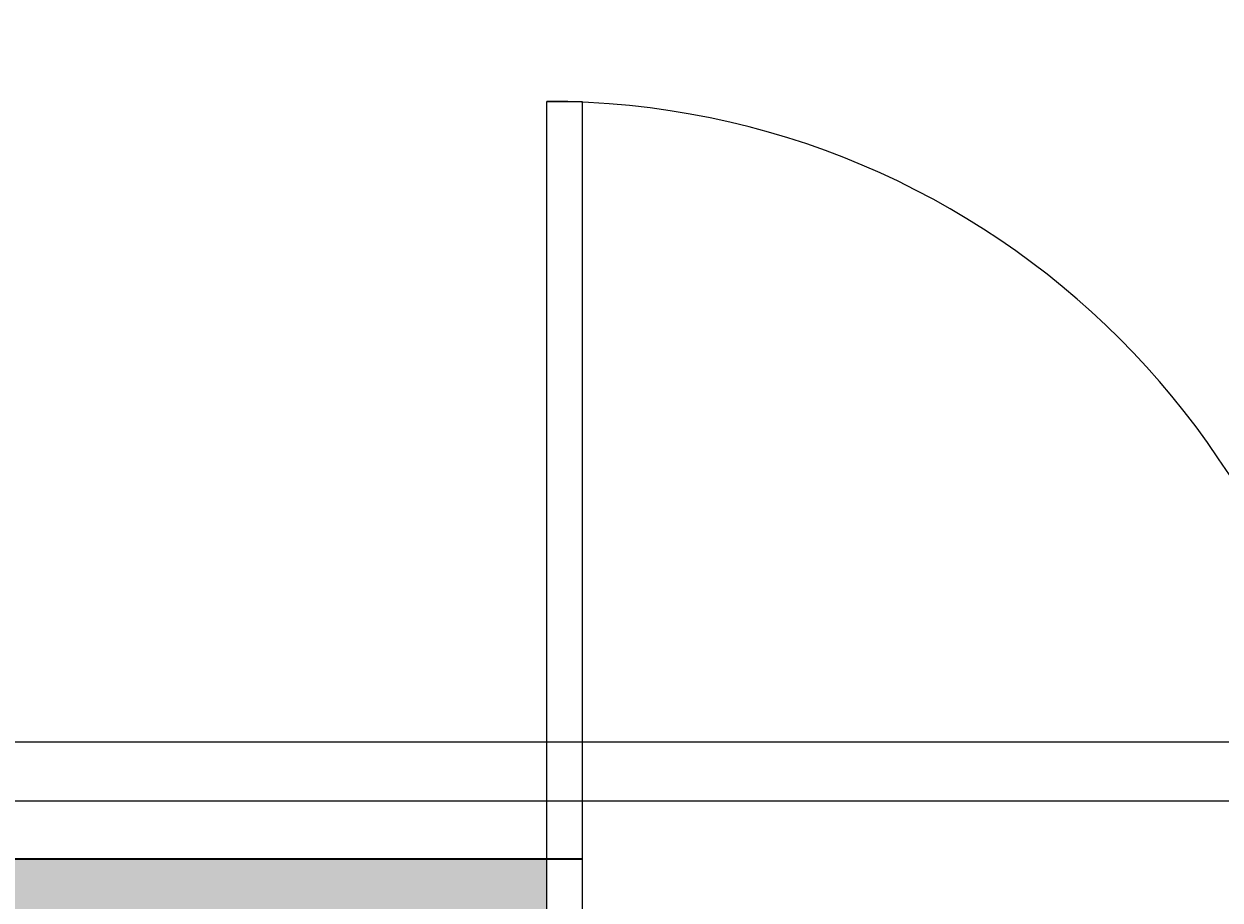
# Model space of a CAD drawing. Units: inches. Extents: x 1998 to 2588, y 1139 to 1977.
# Tile 48 of 134: x 2282 to 2313, y 1592 to 1615. Entities that reach past the tile are written whole.
import ezdxf

# ---------------------------------------------------------------- set-up
doc = ezdxf.new("R2010")
doc.units = ezdxf.units.IN
for name, color, linetype, lineweight in [('A-ANNO-DIMS', 2, 'Continuous', 18), ('A-WALL-PATT', 252, 'Continuous', 13), ('DOOR', 52, 'Continuous', 25), ('WALL', 200, 'Continuous', 35)]:
    doc.layers.add(name, color=color, linetype=linetype, lineweight=lineweight)
doc.styles.get("Standard").update_dxf_attribs({"font": 'arial.ttf'})
doc.dimstyles.get("Standard").update_dxf_attribs({"dimtxt": 0.18, "dimasz": 0.18, "dimexe": 0.18, "dimexo": 0.0625, "dimgap": 0.09, "dimtad": 0, "dimtih": 1, "dimtoh": 1, "dimdec": 4, "dimzin": 0, "dimdsep": 46, "dimtxsty": 'Standard', "dimcen": 0.09, "dimadec": 0, "dimazin": 0, "dimtfac": 1, "dimtdec": 4, "dimtofl": 0, "dimtmove": 0, "dimatfit": 3, "dimfxl": 1, "dimtolj": 1, "dimtzin": 0, "dimarcsym": 0})

# ---------------------------------------------------------------- blocks, each defined once
blk = doc.blocks.new('*U2')
for p, q in [((0, 0), (0, -6)), ((40, 0), (40, -6))]:
    blk.add_line(p, q)
blk.add_lwpolyline([(0, 0), (0, 40), (1.75, 40), (1.75, 0)], close=True)
blk.add_arc((0, 0), 40, 0, 90)
blk = doc.blocks.new('*D30')
at = {"layer": 'A-ANNO-DIMS', "color": 0, "lineweight": -2, "transparency": 16777216}
for p, q in [((2407.91, 1636.732), (1997.843, 1636.732)), ((1998.023, 1636.552), (1998.023, 1615.913)), ((1998.023, 1594.912), (1998.023, 1615.552)), ((2407.91, 1594.732), (1997.843, 1594.732))]:
    blk.add_line(p, q, dxfattribs=at)
at = {"layer": 'A-ANNO-DIMS', "color": 0, "transparency": 16777216}
for points in [[(1997.993, 1636.552), (1998.053, 1636.552), (1998.023, 1636.732)], [(1997.993, 1594.912), (1998.053, 1594.912), (1998.023, 1594.732)]]:
    blk.add_solid(points, dxfattribs=at)
at = {"layer": 'Defpoints', "color": 0, "transparency": 16777216}
for p in [(1998.023, 1636.732), (2407.973, 1636.732), (2407.973, 1594.732)]:
    blk.add_point(p, dxfattribs=at)
at = {"layer": 'A-ANNO-DIMS', "color": 0, "transparency": 16777216, "insert": (1998.023, 1615.732), "char_height": 0.18, "attachment_point": 5}
blk.add_mtext('\\A1;42', dxfattribs=at)
blk = doc.blocks.new('*D34')
at = {"layer": 'A-ANNO-DIMS', "color": 0, "lineweight": -2, "transparency": 16777216}
for p, q in [((2407.91, 1594.732), (1997.843, 1594.732)), ((1998.023, 1594.552), (1998.023, 1558.913)), ((1998.023, 1522.912), (1998.023, 1558.552)), ((2407.91, 1522.732), (1997.843, 1522.732))]:
    blk.add_line(p, q, dxfattribs=at)
at = {"layer": 'A-ANNO-DIMS', "color": 0, "transparency": 16777216}
for points in [[(1997.993, 1594.552), (1998.053, 1594.552), (1998.023, 1594.732)], [(1997.993, 1522.912), (1998.053, 1522.912), (1998.023, 1522.732)]]:
    blk.add_solid(points, dxfattribs=at)
at = {"layer": 'Defpoints', "color": 0, "transparency": 16777216}
for p in [(1998.023, 1594.732), (2407.973, 1594.732), (2407.973, 1522.732)]:
    blk.add_point(p, dxfattribs=at)
at = {"layer": 'A-ANNO-DIMS', "color": 0, "transparency": 16777216, "insert": (1998.023, 1558.732), "char_height": 0.18, "attachment_point": 5}
blk.add_mtext('\\A1;72', dxfattribs=at)
blk = doc.blocks.new('*D39')
at = {"layer": 'A-ANNO-DIMS', "color": 0, "lineweight": -2, "transparency": 16777216}
for p, q in [((2115.035, 1628.742), (2588.309, 1628.742)), ((2588.129, 1628.562), (2588.129, 1612.685)), ((2588.129, 1596.444), (2588.129, 1612.321)), ((2115.035, 1596.264), (2588.309, 1596.264))]:
    blk.add_line(p, q, dxfattribs=at)
at = {"layer": 'A-ANNO-DIMS', "color": 0, "transparency": 16777216}
for points in [[(2588.099, 1628.562), (2588.159, 1628.562), (2588.129, 1628.742)], [(2588.099, 1596.444), (2588.159, 1596.444), (2588.129, 1596.264)]]:
    blk.add_solid(points, dxfattribs=at)
at = {"layer": 'Defpoints', "color": 0, "transparency": 16777216}
for p in [(2114.973, 1628.742), (2588.129, 1628.742), (2114.973, 1596.264)]:
    blk.add_point(p, dxfattribs=at)
at = {"layer": 'A-ANNO-DIMS', "color": 0, "transparency": 16777216, "insert": (2588.129, 1612.503), "char_height": 0.18, "attachment_point": 5}
blk.add_mtext('\\A1;32.48', dxfattribs=at)

msp = doc.modelspace()

# ---------------------------------------------------------------- hatches: boundary and pattern name
at = {"layer": 'A-WALL-PATT'}
h = msp.add_hatch(color=256, dxfattribs=at)
h.dxf.hatch_style = 1
h.paths.add_polyline_path([(2222.9729, 1888.7324), (2099.4125, 1888.7324), (2099.4125, 1879.7324), (2222.9729, 1879.7324)])
h.paths.add_polyline_path([(2096.9729, 1868.3278), (2087.9729, 1868.3278), (2087.9729, 1775.637), (2096.9729, 1775.637)])
h.paths.add_polyline_path([(2227.4729, 1868.3278), (2222.9729, 1868.3278), (2222.9729, 1774.3318), (2227.4729, 1774.3318)])
h.paths.add_polyline_path([(2188.3019, 1759.7324), (2138.6074, 1759.7324), (2099.4125, 1759.7324), (2099.4125, 1755.2324), (2176.9729, 1755.2324), (2188.3019, 1755.2324)])
h.paths.add_polyline_path([(2087.9729, 1759.7324), (2059.4729, 1759.7324), (2059.4729, 1702.7324), (2087.9729, 1702.7324), (2087.9729, 1707.2324), (2063.9729, 1707.2324), (2063.9729, 1755.2324), (2087.9729, 1755.2324)])
h.paths.add_polyline_path([(2096.9729, 1755.2324), (2087.9729, 1755.2324), (2087.9729, 1707.2324), (2096.9729, 1707.2324)])
h.paths.add_polyline_path([(2187.0461, 1707.2324), (2105.9729, 1707.2324), (2096.9729, 1707.2324), (2087.9729, 1707.2324), (2087.9729, 1702.7324), (2105.9729, 1702.7324), (2114.9729, 1702.7324), (2187.0461, 1702.7324)])
h.paths.add_polyline_path([(2181.4729, 1719.2028), (2176.9729, 1719.2028), (2176.9729, 1707.2324), (2181.4729, 1707.2324)])
h.paths.add_polyline_path([(2216.0332, 1588.7324), (2114.9729, 1588.7324), (2105.9729, 1588.7324), (2105.9729, 1584.2324), (2216.0332, 1584.2324)])
h.paths.add_polyline_path([(2077.691, 1588.7324), (2061.4729, 1588.7324), (2061.4729, 1584.2324), (2077.691, 1584.2324)])
h.paths.add_polyline_path([(2105.9729, 1588.7324), (2098.0956, 1588.7324), (2098.0956, 1584.2324), (2105.9729, 1584.2324)])
h.paths.add_polyline_path([(2114.9729, 1596.2642), (2110.1012, 1596.2642), (2105.9729, 1596.2642), (2105.9729, 1588.7324), (2114.9729, 1588.7324)])
h.paths.add_polyline_path([(2114.9729, 1584.2324), (2105.9729, 1584.2324), (2105.9729, 1580.249), (2110.1012, 1580.249), (2114.9729, 1580.249)])
h.paths.add_polyline_path([(2114.9729, 1547.7716), (2110.1012, 1547.7716, -0.0318759), (2105.9729, 1548.035), (2105.9729, 1470.2324), (2108.3775, 1470.2324), (2108.3775, 1465.7324), (2186.2943, 1465.7324), (2186.2943, 1470.2324), (2114.9729, 1470.2324)])
h.paths.add_polyline_path([(2227.4729, 1584.2324), (2222.9729, 1584.2324), (2222.9729, 1486.137), (2227.4729, 1486.137)])
h.paths.add_polyline_path([(2295.4138, 1593.2324), (2227.4729, 1593.2324), (2227.4729, 1588.7324), (2295.4138, 1588.7324), (2295.4138, 1591.8729)])
h.paths.add_polyline_path([(2345.9729, 1627.1165), (2341.4729, 1627.1165), (2341.4729, 1593.2324), (2337.2869, 1593.2324), (2337.2869, 1591.8729), (2337.2869, 1588.7324), (2345.9729, 1588.7324)])
h.paths.add_polyline_path([(2291.9729, 1588.7324), (2287.4729, 1588.7324), (2287.4729, 1522.7324), (2291.9729, 1522.7324)])
h.paths.add_polyline_path([(2291.9729, 1522.7324), (2287.4729, 1522.7324), (2227.4729, 1522.7324), (2227.4729, 1518.2324), (2291.9729, 1518.2324)])
h.paths.add_polyline_path([(2295.7347, 1519.5919), (2295.7347, 1522.7324), (2291.9729, 1522.7324), (2291.9729, 1518.2324), (2295.7347, 1518.2324)])
h.paths.add_polyline_path([(2345.9729, 1522.7324), (2337.6078, 1522.7324), (2337.6078, 1519.5919), (2337.6078, 1518.2324), (2341.4729, 1518.2324), (2341.4729, 1488.5616), (2345.9729, 1488.5616)])
h.paths.add_polyline_path([(2345.9729, 1468.1569), (2341.4729, 1468.1569), (2341.4729, 1374.2324), (2227.4729, 1374.2324), (2227.4729, 1369.7324), (2345.9729, 1369.7324)])
h.paths.add_polyline_path([(2345.9729, 1369.7324), (2341.4729, 1369.7324), (2341.4729, 1362.2324), (2345.9729, 1362.2324)])
h.paths.add_polyline_path([(2345.9729, 1317.7324), (2345.9729, 1322.2324), (2341.4729, 1322.2324), (2341.4729, 1285.137), (2345.9729, 1285.137)], flags=17)
h.paths.add_polyline_path([(2356.2096, 1322.2324), (2345.9729, 1322.2324), (2345.9729, 1317.7324), (2356.2096, 1317.7324), (2356.2096, 1319.3088)], flags=17)
h.paths.add_polyline_path([(2393.9729, 1322.2324), (2375.6999, 1322.2324), (2375.6999, 1319.3088, -0.0202458), (2375.636, 1317.7324), (2393.9729, 1317.7324)], flags=17)
h.paths.add_polyline_path([(2398.4729, 1322.2324), (2393.9729, 1322.2324), (2393.9729, 1317.7324), (2393.9729, 1237.7324), (2345.9729, 1237.7324), (2345.9729, 1264.7324), (2341.4729, 1264.7324), (2341.4729, 1228.7324), (2393.9729, 1228.7324), (2482.7412, 1228.7324), (2482.7412, 1237.7324), (2398.4729, 1237.7324), (2398.4729, 1297.1029)])
h.paths.add_polyline_path([(2398.4729, 1362.2324), (2393.9729, 1362.2324), (2393.9729, 1357.7324), (2398.4729, 1357.7324)])
h.paths.add_polyline_path([(2345.9729, 1329.7549), (2341.4729, 1329.7549), (2341.4729, 1322.2324), (2345.9729, 1322.2324)])

# ---------------------------------------------------------------- linework, layer by layer
at = {"layer": 'WALL'}
msp.add_line((2296.3298, 1593.2324), (2227.4729, 1593.2324), dxfattribs=at)

# ---------------------------------------------------------------- block references
at = {"layer": 'DOOR', "xscale": 0.5234138920659225, "yscale": 0.5234138920659225, "zscale": 0.5234138920659225}
msp.add_blockref('*U2', (2295.4138, 1591.8729), dxfattribs=at)

# ---------------------------------------------------------------- dimensions: what is measured, and where the dimension line sits
at = {"layer": 'A-ANNO-DIMS'}
for base, p1, p2, override, picture, middle in [((1998.0229, 1636.7324), (2407.9729, 1594.7324), (2407.9729, 1636.7324), {"dimdec": 0, "dimlfac": 1, "dimrnd": 0, "dimzin": 0, "dimdsep": 46, "dimlunit": 2}, '*D30', (1998.0229, 1615.7324)), ((2588.1286, 1628.7416), (2114.9729, 1596.2642), (2114.9729, 1628.7416), {"dimdec": 2, "dimlfac": 1, "dimrnd": 0, "dimzin": 0, "dimdsep": 46, "dimlunit": 2}, '*D39', (2588.1286, 1612.5029)), ((1998.0229, 1594.7324), (2407.9729, 1522.7324), (2407.9729, 1594.7324), {"dimdec": 0, "dimlfac": 1, "dimrnd": 0, "dimzin": 0, "dimdsep": 46, "dimlunit": 2}, '*D34', (1998.0229, 1558.7324))]:
    dim = msp.add_linear_dim(base=base, p1=p1, p2=p2, angle=90, dimstyle='Standard', override=override, dxfattribs=at)
    dim.commit()
    dim.dimension.update_dxf_attribs({"geometry": picture, "text_midpoint": middle})

doc.saveas('drawing.dxf')
